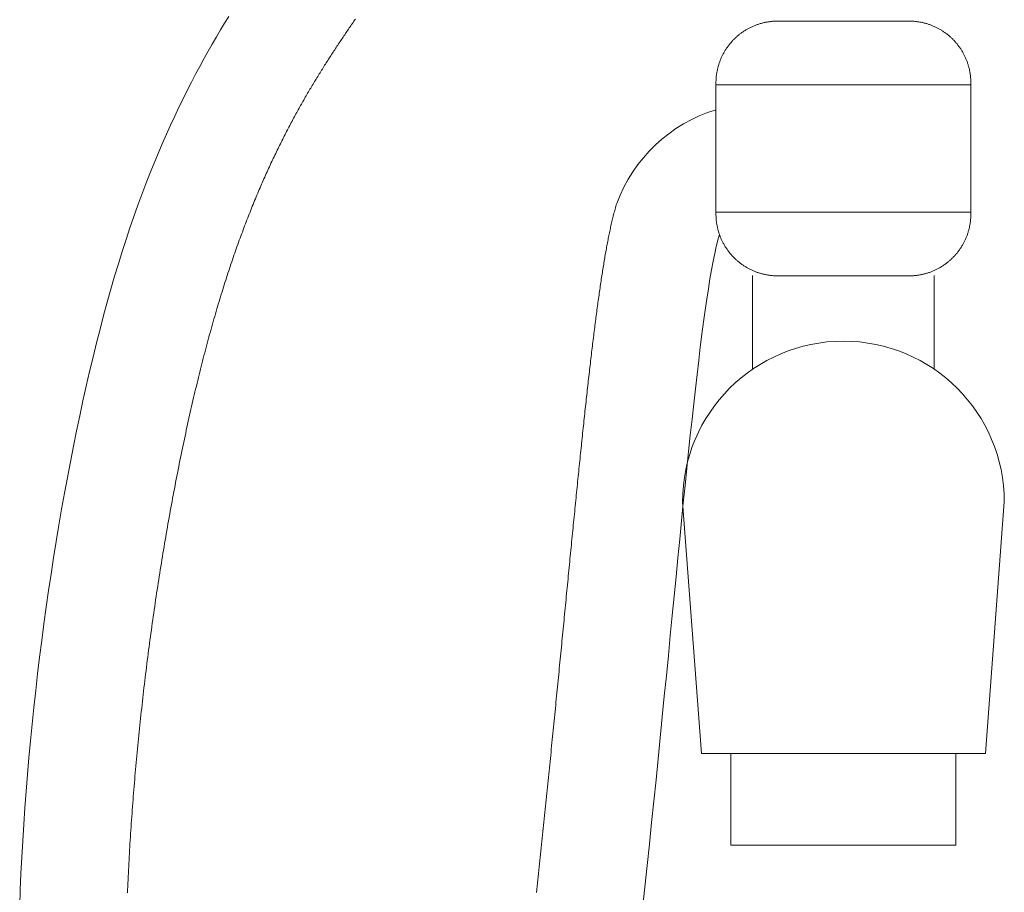
# Model space of a CAD drawing. Units: inches. Extents: x 64 to 1167, y 117 to 939.
# Tile 31 of 56: x 1044.26 to 1050.377, y 448.409 to 453.834. Entities that reach past the tile are written whole.
import ezdxf

# ---------------------------------------------------------------- set-up
doc = ezdxf.new("R2010")
doc.units = ezdxf.units.IN
doc.header["$MEASUREMENT"] = 0
doc.layers.add('A-FLOR-FIXT', color=8, linetype='Continuous', lineweight=18)

# ---------------------------------------------------------------- blocks, each defined once
blk = doc.blocks.new('A$C01277C2D')
for p, q in [((4.1384, 8.1142), (3.5444, 8.1142)), ((4.4355, 7.8172), (3.2473, 7.8172)), ((3.2473, 7.8172), (3.2473, 7.2231)), ((4.4355, 7.2231), (4.4355, 7.8172)), ((3.2473, 7.2231), (4.4355, 7.2231)), ((3.4178, 6.4903), (3.4178, 6.9283)), ((3.5444, 6.9261), (4.1384, 6.9261)), ((4.265, 6.4903), (4.265, 6.9283)), ((3.0914, 5.8714), (3.1791, 4.6978)), ((4.5914, 5.8714), (4.5038, 4.6978)), ((3.1791, 4.6978), (4.5038, 4.6978)), ((3.3169, 4.271), (3.3169, 4.6978)), ((4.366, 4.271), (4.366, 4.6978)), ((3.3169, 4.271), (4.366, 4.271))]:
    blk.add_line(p, q)
for points in [[(3.2634, 7.1191, 0), (3.2561, 7.0931, 0), (3.2487, 7.0635, 0), (3.2414, 7.0306, 0), (3.234, 6.9943, 0), (3.2267, 6.9547, 0), (3.2193, 6.912, 0), (3.2119, 6.8662, 0), (3.2044, 6.8175, 0), (3.197, 6.7657, 0), (3.1895, 6.7112, 0), (3.1819, 6.6539, 0), (3.1743, 6.594, 0), (3.1667, 6.5315, 0), (3.159, 6.4665, 0), (3.1512, 6.399, 0), (3.1434, 6.3293, 0), (3.1355, 6.2573, 0), (3.1276, 6.1831, 0), (3.1195, 6.1069, 0), (3.1114, 6.0287, 0), (3.1033, 5.9486, 0), (3.095, 5.8666, 0), (3.0866, 5.7829, 0), (3.0781, 5.6976, 0), (3.0696, 5.6107, 0), (3.0609, 5.5222, 0), (3.0522, 5.4324, 0), (3.0433, 5.3413, 0), (3.0343, 5.2489, 0), (3.0252, 5.1554, 0), (3.0159, 5.0608, 0), (3.0065, 4.9653, 0), (2.9971, 4.8688, 0), (2.9874, 4.7715, 0), (2.9776, 4.6735, 0), (2.9677, 4.5748, 0), (2.9577, 4.4756, 0), (2.9474, 4.3758, 0), (2.9371, 4.2757, 0), (2.9265, 4.1753, 0), (2.9158, 4.0746, 0), (2.9049, 3.9738, 0)], [(0.0012, 3.9867, 0), (0.004, 4.0619, 0), (0.0072, 4.1376, 0), (0.011, 4.2138, 0), (0.0153, 4.2904, 0), (0.0201, 4.3674, 0), (0.0254, 4.4448, 0), (0.0312, 4.5224, 0), (0.0375, 4.6002, 0), (0.0443, 4.6783, 0), (0.0515, 4.7564, 0), (0.0592, 4.8347, 0), (0.0673, 4.9129, 0), (0.0759, 4.9912, 0), (0.0849, 5.0694, 0), (0.0943, 5.1475, 0), (0.1041, 5.2255, 0), (0.1144, 5.3032, 0), (0.125, 5.3807, 0), (0.1361, 5.4579, 0), (0.1475, 5.5347, 0), (0.1593, 5.6112, 0), (0.1715, 5.6872, 0), (0.184, 5.7627, 0), (0.1969, 5.8377, 0), (0.2101, 5.9121, 0), (0.2237, 5.9858, 0), (0.2375, 6.0589, 0), (0.2517, 6.1312, 0), (0.2663, 6.2027, 0), (0.2811, 6.2734, 0), (0.2962, 6.3433, 0), (0.3116, 6.4122, 0), (0.3272, 6.4801, 0), (0.3432, 6.547, 0), (0.3594, 6.6129, 0), (0.3758, 6.6776, 0), (0.3925, 6.7411, 0), (0.4095, 6.8035, 0), (0.4266, 6.8645, 0), (0.444, 6.9243, 0), (0.4616, 6.9827, 0), (0.4794, 7.0398, 0), (0.4974, 7.0955, 0), (0.5155, 7.15, 0), (0.5339, 7.2032, 0), (0.5524, 7.2552, 0), (0.571, 7.3059, 0), (0.5898, 7.3555, 0), (0.6086, 7.4039, 0), (0.6276, 7.4512, 0), (0.6467, 7.4973, 0), (0.6659, 7.5424, 0), (0.6852, 7.5864, 0), (0.7045, 7.6293, 0), (0.7239, 7.6713, 0), (0.7433, 7.7122, 0), (0.7628, 7.7522, 0), (0.7822, 7.7913, 0), (0.8017, 7.8294, 0), (0.8212, 7.8667, 0), (0.8407, 7.9031, 0), (0.8601, 7.9386, 0), (0.8795, 7.9734, 0), (0.8989, 8.0074, 0), (0.9182, 8.0405, 0), (0.9374, 8.073, 0), (0.9566, 8.1047, 0), (0.9757, 8.1358, 0)], [(0.5038, 4.0475, 0), (0.5044, 4.0627, 0), (0.5051, 4.078, 0), (0.5057, 4.0932, 0), (0.5064, 4.1085, 0), (0.5071, 4.1238, 0), (0.5079, 4.1391, 0), (0.5086, 4.1545, 0), (0.5094, 4.1698, 0), (0.5102, 4.1852, 0), (0.511, 4.2007, 0), (0.5119, 4.2161, 0), (0.5127, 4.2316, 0), (0.5136, 4.2471, 0), (0.5145, 4.2626, 0), (0.5155, 4.2781, 0), (0.5164, 4.2937, 0), (0.5174, 4.3092, 0), (0.5184, 4.3248, 0), (0.5194, 4.3404, 0), (0.5205, 4.356, 0), (0.5215, 4.3717, 0), (0.5226, 4.3873, 0), (0.5237, 4.403, 0), (0.5249, 4.4187, 0), (0.526, 4.4344, 0), (0.5272, 4.4501, 0), (0.5284, 4.4658, 0), (0.5296, 4.4815, 0), (0.5308, 4.4973, 0), (0.5321, 4.513, 0), (0.5333, 4.5288, 0), (0.5346, 4.5446, 0), (0.5359, 4.5604, 0), (0.5373, 4.5762, 0), (0.5386, 4.592, 0), (0.54, 4.6078, 0), (0.5414, 4.6237, 0), (0.5428, 4.6395, 0), (0.5443, 4.6554, 0), (0.5457, 4.6712, 0), (0.5472, 4.6871, 0), (0.5487, 4.703, 0), (0.5502, 4.7188, 0), (0.5517, 4.7347, 0), (0.5533, 4.7506, 0), (0.5549, 4.7665, 0), (0.5564, 4.7824, 0), (0.5581, 4.7983, 0), (0.5597, 4.8141, 0), (0.5613, 4.83, 0), (0.563, 4.8459, 0), (0.5647, 4.8618, 0), (0.5664, 4.8777, 0), (0.5681, 4.8937, 0), (0.5699, 4.9096, 0), (0.5716, 4.9254, 0), (0.5734, 4.9413, 0), (0.5752, 4.9572, 0), (0.577, 4.9731, 0), (0.5789, 4.989, 0), (0.5807, 5.0049, 0), (0.5826, 5.0208, 0), (0.5845, 5.0367, 0), (0.5864, 5.0526, 0), (0.5883, 5.0684, 0), (0.5903, 5.0843, 0), (0.5922, 5.1001, 0), (0.5942, 5.116, 0), (0.5962, 5.1318, 0), (0.5982, 5.1477, 0), (0.6003, 5.1635, 0), (0.6023, 5.1793, 0), (0.6044, 5.1951, 0), (0.6065, 5.2109, 0), (0.6086, 5.2267, 0), (0.6107, 5.2425, 0), (0.6128, 5.2582, 0), (0.615, 5.274, 0), (0.6172, 5.2897, 0), (0.6194, 5.3055, 0), (0.6216, 5.3212, 0), (0.6238, 5.3369, 0), (0.626, 5.3525, 0), (0.6283, 5.3682, 0), (0.6306, 5.3839, 0), (0.6328, 5.3995, 0), (0.6351, 5.4151, 0), (0.6375, 5.4307, 0), (0.6398, 5.4463, 0), (0.6422, 5.4619, 0), (0.6445, 5.4775, 0), (0.6469, 5.493, 0), (0.6493, 5.5085, 0), (0.6517, 5.524, 0), (0.6542, 5.5395, 0), (0.6566, 5.5549, 0), (0.6591, 5.5704, 0), (0.6616, 5.5858, 0), (0.664, 5.6012, 0), (0.6666, 5.6165, 0), (0.6691, 5.6319, 0), (0.6716, 5.6472, 0), (0.6742, 5.6625, 0), (0.6767, 5.6778, 0), (0.6793, 5.693, 0), (0.6819, 5.7082, 0), (0.6845, 5.7234, 0), (0.6872, 5.7386, 0), (0.6898, 5.7537, 0), (0.6925, 5.7688, 0), (0.6951, 5.7839, 0), (0.6978, 5.799, 0), (0.7005, 5.814, 0), (0.7032, 5.829, 0), (0.7059, 5.8439, 0), (0.7087, 5.8589, 0), (0.7114, 5.8738, 0), (0.7142, 5.8886, 0), (0.717, 5.9035, 0), (0.7197, 5.9183, 0), (0.7225, 5.933, 0), (0.7254, 5.9478, 0), (0.7282, 5.9625, 0), (0.731, 5.9771, 0), (0.7339, 5.9918, 0), (0.7368, 6.0064, 0), (0.7396, 6.0209, 0), (0.7425, 6.0354, 0), (0.7454, 6.0499, 0), (0.7483, 6.0644, 0), (0.7513, 6.0788, 0), (0.7542, 6.0931, 0), (0.7572, 6.1075, 0), (0.7601, 6.1217, 0), (0.7631, 6.136, 0), (0.7661, 6.1502, 0), (0.7691, 6.1643, 0), (0.7721, 6.1785, 0), (0.7751, 6.1925, 0), (0.7781, 6.2066, 0), (0.7812, 6.2206, 0), (0.7842, 6.2345, 0), (0.7873, 6.2484, 0), (0.7904, 6.2622, 0), (0.7934, 6.2761, 0), (0.7965, 6.2898, 0), (0.7996, 6.3035, 0), (0.8027, 6.3172, 0), (0.8059, 6.3308, 0), (0.809, 6.3444, 0), (0.8122, 6.3579, 0), (0.8153, 6.3714, 0), (0.8185, 6.3848, 0), (0.8216, 6.3982, 0), (0.8248, 6.4115, 0), (0.828, 6.4247, 0), (0.8312, 6.4379, 0), (0.8344, 6.4511, 0), (0.8377, 6.4642, 0), (0.8409, 6.4772, 0), (0.8441, 6.4902, 0), (0.8474, 6.5031, 0), (0.8506, 6.516, 0), (0.8539, 6.5287, 0), (0.8571, 6.5415, 0), (0.8604, 6.5541, 0), (0.8637, 6.5667, 0), (0.867, 6.5793, 0), (0.8703, 6.5917, 0), (0.8736, 6.6042, 0), (0.8769, 6.6165, 0), (0.8802, 6.6288, 0), (0.8835, 6.6411, 0), (0.8869, 6.6532, 0), (0.8902, 6.6654, 0), (0.8935, 6.6774, 0), (0.8969, 6.6894, 0), (0.9002, 6.7013, 0), (0.9036, 6.7132, 0), (0.907, 6.7251, 0), (0.9104, 6.7368, 0), (0.9137, 6.7485, 0), (0.9171, 6.7602, 0), (0.9205, 6.7717, 0), (0.9239, 6.7832, 0), (0.9273, 6.7947, 0), (0.9308, 6.8061, 0), (0.9342, 6.8175, 0), (0.9376, 6.8287, 0), (0.941, 6.8399, 0), (0.9445, 6.8511, 0), (0.9479, 6.8622, 0), (0.9514, 6.8733, 0), (0.9548, 6.8843, 0), (0.9583, 6.8952, 0), (0.9618, 6.906, 0), (0.9652, 6.9169, 0), (0.9687, 6.9276, 0), (0.9722, 6.9383, 0), (0.9757, 6.9489, 0), (0.9792, 6.9595, 0), (0.9827, 6.97, 0), (0.9862, 6.9805, 0), (0.9897, 6.9909, 0), (0.9932, 7.0012, 0), (0.9967, 7.0115, 0), (1.0002, 7.0218, 0), (1.0037, 7.0319, 0), (1.0073, 7.042, 0), (1.0108, 7.0521, 0), (1.0143, 7.0621, 0), (1.0179, 7.072, 0), (1.0214, 7.0819, 0), (1.025, 7.0918, 0), (1.0285, 7.1015, 0), (1.0321, 7.1112, 0), (1.0356, 7.1209, 0), (1.0392, 7.1305, 0), (1.0428, 7.14, 0), (1.0463, 7.1495, 0), (1.0499, 7.159, 0), (1.0535, 7.1683, 0), (1.0571, 7.1777, 0), (1.0607, 7.187, 0), (1.0642, 7.1962, 0), (1.0678, 7.2054, 0), (1.0714, 7.2145, 0), (1.075, 7.2236, 0), (1.0786, 7.2326, 0), (1.0822, 7.2416, 0), (1.0858, 7.2505, 0), (1.0894, 7.2594, 0), (1.093, 7.2683, 0), (1.0966, 7.277, 0), (1.1002, 7.2858, 0), (1.1038, 7.2945, 0), (1.1075, 7.3031, 0), (1.1111, 7.3117, 0), (1.1147, 7.3203, 0), (1.1183, 7.3288, 0), (1.1219, 7.3372, 0), (1.1256, 7.3456, 0), (1.1292, 7.354, 0), (1.1328, 7.3623, 0), (1.1364, 7.3706, 0), (1.1401, 7.3788, 0), (1.1437, 7.387, 0), (1.1473, 7.3951, 0), (1.151, 7.4032, 0), (1.1546, 7.4113, 0), (1.1582, 7.4193, 0), (1.1619, 7.4273, 0), (1.1655, 7.4352, 0), (1.1691, 7.4431, 0), (1.1728, 7.4509, 0), (1.1764, 7.4587, 0), (1.1801, 7.4665, 0), (1.1837, 7.4742, 0), (1.1873, 7.4819, 0), (1.191, 7.4895, 0), (1.1946, 7.4971, 0), (1.1983, 7.5046, 0), (1.2019, 7.5122, 0), (1.2056, 7.5196, 0), (1.2092, 7.5271, 0), (1.2128, 7.5345, 0), (1.2165, 7.5418, 0), (1.2201, 7.5492, 0), (1.2238, 7.5564, 0), (1.2274, 7.5637, 0), (1.2311, 7.5709, 0), (1.2347, 7.5781, 0), (1.2384, 7.5852, 0), (1.242, 7.5923, 0), (1.2456, 7.5994, 0), (1.2493, 7.6064, 0), (1.2529, 7.6134, 0), (1.2566, 7.6203, 0), (1.2602, 7.6273, 0), (1.2638, 7.6341, 0), (1.2675, 7.641, 0), (1.2711, 7.6478, 0), (1.2748, 7.6546, 0), (1.2784, 7.6614, 0), (1.282, 7.6681, 0), (1.2856, 7.6748, 0), (1.2893, 7.6814, 0), (1.2929, 7.688, 0), (1.2965, 7.6946, 0), (1.3002, 7.7012, 0), (1.3038, 7.7077, 0), (1.3074, 7.7142, 0), (1.3111, 7.7207, 0), (1.3147, 7.7271, 0), (1.3183, 7.7336, 0), (1.3219, 7.7399, 0), (1.3256, 7.7463, 0), (1.3292, 7.7526, 0), (1.3328, 7.7589, 0), (1.3364, 7.7652, 0), (1.34, 7.7714, 0), (1.3437, 7.7776, 0), (1.3473, 7.7838, 0), (1.3509, 7.79, 0), (1.3545, 7.7961, 0), (1.3581, 7.8022, 0), (1.3617, 7.8083, 0), (1.3653, 7.8143, 0), (1.3689, 7.8204, 0), (1.3726, 7.8264, 0), (1.3762, 7.8324, 0), (1.3798, 7.8383, 0), (1.3834, 7.8442, 0), (1.387, 7.8502, 0), (1.3906, 7.8561, 0), (1.3942, 7.8619, 0), (1.3978, 7.8678, 0), (1.4014, 7.8736, 0), (1.405, 7.8794, 0), (1.4086, 7.8852, 0), (1.4122, 7.8909, 0), (1.4158, 7.8967, 0), (1.4194, 7.9024, 0), (1.423, 7.9081, 0), (1.4266, 7.9138, 0), (1.4302, 7.9194, 0), (1.4338, 7.9251, 0), (1.4374, 7.9307, 0), (1.441, 7.9363, 0), (1.4446, 7.9419, 0), (1.4482, 7.9475, 0), (1.4518, 7.953, 0), (1.4554, 7.9586, 0), (1.459, 7.9641, 0), (1.4626, 7.9696, 0), (1.4661, 7.9751, 0), (1.4697, 7.9806, 0), (1.4733, 7.986, 0), (1.4769, 7.9915, 0), (1.4805, 7.9969, 0), (1.4841, 8.0023, 0), (1.4876, 8.0077, 0), (1.4912, 8.0131, 0), (1.4948, 8.0185, 0), (1.4984, 8.0239, 0), (1.502, 8.0292, 0), (1.5055, 8.0346, 0), (1.5091, 8.0399, 0), (1.5127, 8.0452, 0), (1.5163, 8.0505, 0), (1.5198, 8.0558, 0), (1.5234, 8.0611, 0), (1.527, 8.0664, 0), (1.5306, 8.0717, 0), (1.5341, 8.0769, 0), (1.5377, 8.0822, 0), (1.5413, 8.0874, 0), (1.5448, 8.0927, 0), (1.5484, 8.0979, 0), (1.552, 8.1031, 0), (1.5555, 8.1083, 0), (1.5591, 8.1135, 0), (1.5627, 8.1187, 0), (1.5662, 8.1239, 0)], [(3.2474, 7.8172, 0), (3.2473, 7.8209, 0), (3.2472, 7.8245, 0), (3.2472, 7.8282, 0), (3.2473, 7.8319, 0), (3.2474, 7.8356, 0), (3.2475, 7.8392, 0), (3.2477, 7.8429, 0), (3.248, 7.8466, 0), (3.2482, 7.8502, 0), (3.2486, 7.8539, 0), (3.2489, 7.8576, 0), (3.2494, 7.8612, 0), (3.2498, 7.8648, 0), (3.2504, 7.8685, 0), (3.2509, 7.8721, 0), (3.2515, 7.8758, 0), (3.2522, 7.8794, 0), (3.2529, 7.883, 0), (3.2536, 7.8866, 0), (3.2544, 7.8902, 0), (3.2553, 7.8937, 0), (3.2562, 7.8973, 0), (3.2571, 7.9009, 0), (3.2581, 7.9044, 0), (3.2591, 7.9079, 0), (3.2602, 7.9115, 0), (3.2613, 7.915, 0), (3.2624, 7.9185, 0), (3.2636, 7.9219, 0), (3.2649, 7.9254, 0), (3.2662, 7.9288, 0), (3.2675, 7.9323, 0), (3.2689, 7.9357, 0), (3.2703, 7.9391, 0), (3.2717, 7.9425, 0), (3.2732, 7.9458, 0), (3.2748, 7.9491, 0), (3.2764, 7.9524, 0), (3.278, 7.9558, 0), (3.2797, 7.959, 0), (3.2814, 7.9623, 0), (3.2832, 7.9655, 0), (3.285, 7.9687, 0), (3.2868, 7.9719, 0), (3.2887, 7.9751, 0), (3.2906, 7.9782, 0), (3.2926, 7.9813, 0), (3.2946, 7.9844, 0), (3.2966, 7.9874, 0), (3.2987, 7.9905, 0), (3.3008, 7.9935, 0), (3.303, 7.9965, 0), (3.3051, 7.9994, 0), (3.3074, 8.0023, 0), (3.3096, 8.0052, 0), (3.3119, 8.0081, 0), (3.3143, 8.0109, 0), (3.3167, 8.0137, 0), (3.3191, 8.0165, 0), (3.3215, 8.0193, 0), (3.324, 8.022, 0), (3.3265, 8.0247, 0), (3.3291, 8.0273, 0), (3.3316, 8.0299, 0), (3.3343, 8.0325, 0), (3.3369, 8.0351, 0), (3.3396, 8.0376, 0), (3.3423, 8.0401, 0), (3.3451, 8.0425, 0), (3.3478, 8.0449, 0), (3.3506, 8.0473, 0), (3.3535, 8.0496, 0), (3.3563, 8.0519, 0), (3.3592, 8.0542, 0), (3.3622, 8.0564, 0), (3.3651, 8.0586, 0), (3.3681, 8.0608, 0), (3.3711, 8.0629, 0), (3.3741, 8.065, 0), (3.3772, 8.067, 0), (3.3803, 8.069, 0), (3.3834, 8.071, 0), (3.3865, 8.0729, 0), (3.3897, 8.0748, 0), (3.3929, 8.0766, 0), (3.3961, 8.0784, 0), (3.3993, 8.0802, 0), (3.4026, 8.0819, 0), (3.4058, 8.0836, 0), (3.4091, 8.0852, 0), (3.4124, 8.0868, 0), (3.4158, 8.0883, 0), (3.4191, 8.0898, 0), (3.4225, 8.0913, 0), (3.4259, 8.0927, 0), (3.4293, 8.0941, 0), (3.4327, 8.0954, 0), (3.4362, 8.0967, 0), (3.4396, 8.098, 0), (3.4431, 8.0991, 0), (3.4466, 8.1003, 0), (3.4501, 8.1014, 0), (3.4536, 8.1025, 0), (3.4572, 8.1035, 0), (3.4607, 8.1045, 0), (3.4643, 8.1054, 0), (3.4678, 8.1063, 0), (3.4714, 8.1071, 0), (3.475, 8.1079, 0), (3.4786, 8.1087, 0), (3.4822, 8.1094, 0), (3.4858, 8.11, 0), (3.4895, 8.1106, 0), (3.4931, 8.1112, 0), (3.4967, 8.1117, 0), (3.5004, 8.1122, 0), (3.504, 8.1126, 0), (3.5077, 8.113, 0), (3.5113, 8.1133, 0), (3.515, 8.1136, 0), (3.5187, 8.1139, 0), (3.5223, 8.1141, 0), (3.526, 8.1142, 0), (3.5297, 8.1143, 0), (3.5334, 8.1143, 0), (3.537, 8.1143, 0), (3.5407, 8.1143, 0), (3.5444, 8.1142, 0)], [(4.1384, 8.1142, 0), (4.1421, 8.1143, 0), (4.1458, 8.1143, 0), (4.1494, 8.1143, 0), (4.1531, 8.1143, 0), (4.1568, 8.1142, 0), (4.1605, 8.1141, 0), (4.1641, 8.1139, 0), (4.1678, 8.1136, 0), (4.1715, 8.1133, 0), (4.1751, 8.113, 0), (4.1788, 8.1126, 0), (4.1825, 8.1122, 0), (4.1861, 8.1117, 0), (4.1897, 8.1112, 0), (4.1934, 8.1106, 0), (4.197, 8.11, 0), (4.2006, 8.1094, 0), (4.2042, 8.1087, 0), (4.2078, 8.1079, 0), (4.2114, 8.1071, 0), (4.215, 8.1063, 0), (4.2186, 8.1054, 0), (4.2221, 8.1045, 0), (4.2257, 8.1035, 0), (4.2292, 8.1025, 0), (4.2327, 8.1014, 0), (4.2362, 8.1003, 0), (4.2397, 8.0991, 0), (4.2432, 8.098, 0), (4.2466, 8.0967, 0), (4.2501, 8.0954, 0), (4.2535, 8.0941, 0), (4.2569, 8.0927, 0), (4.2603, 8.0913, 0), (4.2637, 8.0898, 0), (4.267, 8.0883, 0), (4.2704, 8.0868, 0), (4.2737, 8.0852, 0), (4.277, 8.0836, 0), (4.2803, 8.0819, 0), (4.2835, 8.0802, 0), (4.2867, 8.0784, 0), (4.29, 8.0766, 0), (4.2931, 8.0748, 0), (4.2963, 8.0729, 0), (4.2994, 8.071, 0), (4.3025, 8.069, 0), (4.3056, 8.067, 0), (4.3087, 8.065, 0), (4.3117, 8.0629, 0), (4.3147, 8.0608, 0), (4.3177, 8.0586, 0), (4.3207, 8.0564, 0), (4.3236, 8.0542, 0), (4.3265, 8.0519, 0), (4.3293, 8.0496, 0), (4.3322, 8.0473, 0), (4.335, 8.0449, 0), (4.3378, 8.0425, 0), (4.3405, 8.0401, 0), (4.3432, 8.0376, 0), (4.3459, 8.0351, 0), (4.3486, 8.0325, 0), (4.3512, 8.0299, 0), (4.3537, 8.0273, 0), (4.3563, 8.0247, 0), (4.3588, 8.022, 0), (4.3613, 8.0193, 0), (4.3637, 8.0165, 0), (4.3662, 8.0137, 0), (4.3685, 8.0109, 0), (4.3709, 8.0081, 0), (4.3732, 8.0052, 0), (4.3754, 8.0023, 0), (4.3777, 7.9994, 0), (4.3799, 7.9965, 0), (4.382, 7.9935, 0), (4.3841, 7.9905, 0), (4.3862, 7.9874, 0), (4.3882, 7.9844, 0), (4.3902, 7.9813, 0), (4.3922, 7.9782, 0), (4.3941, 7.9751, 0), (4.396, 7.9719, 0), (4.3978, 7.9687, 0), (4.3996, 7.9655, 0), (4.4014, 7.9623, 0), (4.4031, 7.959, 0), (4.4048, 7.9558, 0), (4.4064, 7.9524, 0), (4.408, 7.9491, 0), (4.4096, 7.9458, 0), (4.4111, 7.9425, 0), (4.4125, 7.9391, 0), (4.4139, 7.9357, 0), (4.4153, 7.9323, 0), (4.4167, 7.9288, 0), (4.4179, 7.9254, 0), (4.4192, 7.9219, 0), (4.4204, 7.9185, 0), (4.4215, 7.915, 0), (4.4227, 7.9115, 0), (4.4237, 7.9079, 0), (4.4247, 7.9044, 0), (4.4257, 7.9009, 0), (4.4267, 7.8973, 0), (4.4275, 7.8937, 0), (4.4284, 7.8902, 0), (4.4292, 7.8866, 0), (4.4299, 7.883, 0), (4.4306, 7.8794, 0), (4.4313, 7.8758, 0), (4.4319, 7.8721, 0), (4.4325, 7.8685, 0), (4.433, 7.8648, 0), (4.4334, 7.8612, 0), (4.4339, 7.8576, 0), (4.4342, 7.8539, 0), (4.4346, 7.8502, 0), (4.4349, 7.8466, 0), (4.4351, 7.8429, 0), (4.4353, 7.8392, 0), (4.4354, 7.8356, 0), (4.4355, 7.8319, 0), (4.4356, 7.8282, 0), (4.4356, 7.8245, 0), (4.4355, 7.8209, 0), (4.4355, 7.8172, 0)], [(2.7847, 7.2636, 0), (2.7827, 7.257, 0), (2.7808, 7.2505, 0), (2.7789, 7.244, 0), (2.7771, 7.2375, 0), (2.7753, 7.231, 0), (2.7735, 7.2245, 0), (2.7718, 7.2181, 0), (2.7701, 7.2116, 0), (2.7685, 7.2052, 0), (2.7668, 7.1988, 0), (2.7652, 7.1923, 0), (2.7637, 7.1859, 0), (2.7621, 7.1794, 0), (2.7606, 7.173, 0), (2.7591, 7.1665, 0), (2.7576, 7.16, 0), (2.7562, 7.1535, 0), (2.7548, 7.147, 0), (2.7534, 7.1405, 0), (2.752, 7.1339, 0), (2.7506, 7.1274, 0), (2.7493, 7.1208, 0), (2.7479, 7.1141, 0), (2.7466, 7.1075, 0), (2.7453, 7.1008, 0), (2.744, 7.0941, 0), (2.7427, 7.0873, 0), (2.7414, 7.0805, 0), (2.7401, 7.0736, 0), (2.7388, 7.0667, 0), (2.7376, 7.0597, 0), (2.7363, 7.0527, 0), (2.735, 7.0457, 0), (2.7337, 7.0386, 0), (2.7325, 7.0314, 0), (2.7312, 7.0242, 0), (2.7299, 7.0169, 0), (2.7287, 7.0096, 0), (2.7274, 7.0023, 0), (2.7262, 6.9949, 0), (2.725, 6.9874, 0), (2.7237, 6.9799, 0), (2.7225, 6.9724, 0), (2.7212, 6.9648, 0), (2.72, 6.9571, 0), (2.7188, 6.9494, 0), (2.7176, 6.9417, 0), (2.7164, 6.9339, 0), (2.7152, 6.926, 0), (2.714, 6.9181, 0), (2.7127, 6.9102, 0), (2.7115, 6.9022, 0), (2.7103, 6.8941, 0), (2.7091, 6.886, 0), (2.7079, 6.8778, 0), (2.7067, 6.8696, 0), (2.7055, 6.8614, 0), (2.7043, 6.8531, 0), (2.7032, 6.8447, 0), (2.702, 6.8363, 0), (2.7008, 6.8278, 0), (2.6996, 6.8193, 0), (2.6984, 6.8107, 0), (2.6972, 6.8021, 0), (2.696, 6.7934, 0), (2.6949, 6.7847, 0), (2.6937, 6.7759, 0), (2.6925, 6.7671, 0), (2.6913, 6.7582, 0), (2.6901, 6.7492, 0), (2.6889, 6.7402, 0), (2.6877, 6.7312, 0), (2.6866, 6.722, 0), (2.6854, 6.7129, 0), (2.6842, 6.7037, 0), (2.683, 6.6944, 0), (2.6818, 6.6851, 0), (2.6806, 6.6757, 0), (2.6795, 6.6663, 0), (2.6783, 6.6568, 0), (2.6771, 6.6473, 0), (2.6759, 6.6377, 0), (2.6747, 6.6281, 0), (2.6735, 6.6184, 0), (2.6723, 6.6087, 0), (2.6712, 6.5989, 0), (2.67, 6.5891, 0), (2.6688, 6.5792, 0), (2.6676, 6.5693, 0), (2.6664, 6.5593, 0), (2.6652, 6.5493, 0), (2.6641, 6.5392, 0), (2.6629, 6.5291, 0), (2.6617, 6.5189, 0), (2.6605, 6.5087, 0), (2.6593, 6.4984, 0), (2.6581, 6.4881, 0), (2.6569, 6.4777, 0), (2.6557, 6.4673, 0), (2.6545, 6.4568, 0), (2.6534, 6.4463, 0), (2.6522, 6.4358, 0), (2.651, 6.4252, 0), (2.6498, 6.4145, 0), (2.6486, 6.4038, 0), (2.6474, 6.3931, 0), (2.6462, 6.3823, 0), (2.645, 6.3715, 0), (2.6438, 6.3606, 0), (2.6426, 6.3496, 0), (2.6414, 6.3387, 0), (2.6402, 6.3277, 0), (2.639, 6.3166, 0), (2.6378, 6.3055, 0), (2.6366, 6.2943, 0), (2.6354, 6.2832, 0), (2.6342, 6.2719, 0), (2.633, 6.2606, 0), (2.6318, 6.2493, 0), (2.6306, 6.2379, 0), (2.6294, 6.2265, 0), (2.6281, 6.2151, 0), (2.6269, 6.2036, 0), (2.6257, 6.192, 0), (2.6245, 6.1805, 0), (2.6233, 6.1688, 0), (2.6221, 6.1571, 0), (2.6208, 6.1454, 0), (2.6196, 6.1337, 0), (2.6184, 6.1219, 0), (2.6172, 6.1101, 0), (2.6159, 6.0982, 0), (2.6147, 6.0863, 0), (2.6135, 6.0743, 0), (2.6122, 6.0623, 0), (2.611, 6.0503, 0), (2.6098, 6.0382, 0), (2.6086, 6.0261, 0), (2.6073, 6.0139, 0), (2.6061, 6.0017, 0), (2.6048, 5.9895, 0), (2.6036, 5.9772, 0), (2.6023, 5.9649, 0), (2.6011, 5.9525, 0), (2.5998, 5.9402, 0), (2.5986, 5.9277, 0), (2.5973, 5.9153, 0), (2.5961, 5.9028, 0), (2.5948, 5.8902, 0), (2.5936, 5.8776, 0), (2.5923, 5.865, 0), (2.5911, 5.8524, 0), (2.5898, 5.8397, 0), (2.5885, 5.827, 0), (2.5873, 5.8142, 0), (2.586, 5.8014, 0), (2.5847, 5.7886, 0), (2.5834, 5.7757, 0), (2.5822, 5.7629, 0), (2.5809, 5.7499, 0), (2.5796, 5.737, 0), (2.5783, 5.724, 0), (2.577, 5.711, 0), (2.5758, 5.6979, 0), (2.5745, 5.6848, 0), (2.5732, 5.6717, 0), (2.5719, 5.6585, 0), (2.5706, 5.6453, 0), (2.5693, 5.6321, 0), (2.568, 5.6189, 0), (2.5667, 5.6056, 0), (2.5654, 5.5923, 0), (2.5641, 5.5789, 0), (2.5628, 5.5656, 0), (2.5615, 5.5522, 0), (2.5602, 5.5387, 0), (2.5588, 5.5253, 0), (2.5575, 5.5118, 0), (2.5562, 5.4983, 0), (2.5549, 5.4847, 0), (2.5536, 5.4712, 0), (2.5522, 5.4576, 0), (2.5509, 5.4439, 0), (2.5496, 5.4303, 0), (2.5482, 5.4166, 0), (2.5469, 5.4029, 0), (2.5456, 5.3891, 0), (2.5442, 5.3754, 0), (2.5429, 5.3616, 0), (2.5415, 5.3478, 0), (2.5402, 5.334, 0), (2.5388, 5.3201, 0), (2.5375, 5.3062, 0), (2.5361, 5.2923, 0), (2.5348, 5.2784, 0), (2.5334, 5.2644, 0), (2.532, 5.2504, 0), (2.5307, 5.2364, 0), (2.5293, 5.2224, 0), (2.528, 5.2083, 0), (2.5266, 5.1942, 0), (2.5252, 5.1801, 0), (2.5238, 5.166, 0), (2.5224, 5.1519, 0), (2.521, 5.1377, 0), (2.5197, 5.1235, 0), (2.5183, 5.1093, 0), (2.5169, 5.0951, 0), (2.5155, 5.0808, 0), (2.5141, 5.0666, 0), (2.5127, 5.0523, 0), (2.5113, 5.038, 0), (2.5099, 5.0237, 0), (2.5085, 5.0093, 0), (2.5071, 4.995, 0), (2.5057, 4.9806, 0), (2.5042, 4.9662, 0), (2.5028, 4.9517, 0), (2.5014, 4.9373, 0), (2.5, 4.9229, 0), (2.4985, 4.9084, 0), (2.4971, 4.8939, 0), (2.4957, 4.8794, 0), (2.4942, 4.8649, 0), (2.4928, 4.8503, 0), (2.4913, 4.8358, 0), (2.4899, 4.8212, 0), (2.4884, 4.8066, 0), (2.487, 4.792, 0), (2.4855, 4.7774, 0), (2.4841, 4.7627, 0), (2.4826, 4.7481, 0), (2.4811, 4.7335, 0), (2.4797, 4.7188, 0), (2.4782, 4.7041, 0), (2.4767, 4.6894, 0), (2.4752, 4.6747, 0), (2.4738, 4.66, 0), (2.4723, 4.6452, 0), (2.4708, 4.6305, 0), (2.4693, 4.6157, 0), (2.4678, 4.6009, 0), (2.4663, 4.5861, 0), (2.4648, 4.5713, 0), (2.4633, 4.5565, 0), (2.4618, 4.5417, 0), (2.4603, 4.5269, 0), (2.4588, 4.5121, 0), (2.4573, 4.4972, 0), (2.4557, 4.4824, 0), (2.4542, 4.4675, 0), (2.4527, 4.4526, 0), (2.4511, 4.4378, 0), (2.4496, 4.4229, 0), (2.4481, 4.408, 0), (2.4465, 4.3931, 0), (2.445, 4.3782, 0), (2.4434, 4.3632, 0), (2.4419, 4.3483, 0), (2.4403, 4.3334, 0), (2.4388, 4.3185, 0), (2.4372, 4.3035, 0), (2.4356, 4.2886, 0), (2.4341, 4.2736, 0), (2.4325, 4.2587, 0), (2.4309, 4.2437, 0), (2.4293, 4.2287, 0), (2.4278, 4.2138, 0), (2.4262, 4.1988, 0), (2.4246, 4.1838, 0), (2.423, 4.1689, 0), (2.4214, 4.1539, 0), (2.4198, 4.1389, 0), (2.4182, 4.1239, 0), (2.4166, 4.1089, 0), (2.415, 4.0939, 0), (2.4133, 4.0789, 0), (2.4117, 4.064, 0), (2.4101, 4.049, 0)], [(3.5444, 6.9261, 0), (3.5407, 6.926, 0), (3.537, 6.926, 0), (3.5334, 6.926, 0), (3.5297, 6.9261, 0), (3.526, 6.9261, 0), (3.5223, 6.9263, 0), (3.5187, 6.9265, 0), (3.515, 6.9267, 0), (3.5113, 6.927, 0), (3.5077, 6.9273, 0), (3.504, 6.9277, 0), (3.5004, 6.9281, 0), (3.4967, 6.9286, 0), (3.4931, 6.9291, 0), (3.4895, 6.9297, 0), (3.4858, 6.9303, 0), (3.4822, 6.931, 0), (3.4786, 6.9317, 0), (3.475, 6.9324, 0), (3.4714, 6.9332, 0), (3.4678, 6.934, 0), (3.4643, 6.9349, 0), (3.4607, 6.9359, 0), (3.4572, 6.9368, 0), (3.4536, 6.9379, 0), (3.4501, 6.9389, 0), (3.4466, 6.94, 0), (3.4431, 6.9412, 0), (3.4396, 6.9424, 0), (3.4362, 6.9436, 0), (3.4327, 6.9449, 0), (3.4293, 6.9463, 0), (3.4259, 6.9476, 0), (3.4225, 6.949, 0), (3.4191, 6.9505, 0), (3.4158, 6.952, 0), (3.4124, 6.9536, 0), (3.4091, 6.9552, 0), (3.4058, 6.9568, 0), (3.4026, 6.9585, 0), (3.3993, 6.9602, 0), (3.3961, 6.9619, 0), (3.3929, 6.9637, 0), (3.3897, 6.9656, 0), (3.3865, 6.9675, 0), (3.3834, 6.9694, 0), (3.3803, 6.9713, 0), (3.3772, 6.9733, 0), (3.3741, 6.9754, 0), (3.3711, 6.9775, 0), (3.3681, 6.9796, 0), (3.3651, 6.9817, 0), (3.3622, 6.9839, 0), (3.3592, 6.9861, 0), (3.3563, 6.9884, 0), (3.3535, 6.9907, 0), (3.3506, 6.9931, 0), (3.3478, 6.9954, 0), (3.3451, 6.9978, 0), (3.3423, 7.0003, 0), (3.3396, 7.0028, 0), (3.3369, 7.0053, 0), (3.3343, 7.0078, 0), (3.3316, 7.0104, 0), (3.3291, 7.013, 0), (3.3265, 7.0157, 0), (3.324, 7.0184, 0), (3.3215, 7.0211, 0), (3.3191, 7.0238, 0), (3.3167, 7.0266, 0), (3.3143, 7.0294, 0), (3.3119, 7.0322, 0), (3.3096, 7.0351, 0), (3.3074, 7.038, 0), (3.3051, 7.0409, 0), (3.303, 7.0439, 0), (3.3008, 7.0469, 0), (3.2987, 7.0499, 0), (3.2966, 7.0529, 0), (3.2946, 7.056, 0), (3.2926, 7.059, 0), (3.2906, 7.0621, 0), (3.2887, 7.0653, 0), (3.2868, 7.0685, 0), (3.285, 7.0716, 0), (3.2832, 7.0748, 0), (3.2814, 7.0781, 0), (3.2797, 7.0813, 0), (3.278, 7.0846, 0), (3.2764, 7.0879, 0), (3.2748, 7.0912, 0), (3.2732, 7.0945, 0), (3.2717, 7.0979, 0), (3.2703, 7.1013, 0), (3.2689, 7.1047, 0), (3.2675, 7.1081, 0), (3.2662, 7.1115, 0), (3.2649, 7.1149, 0), (3.2636, 7.1184, 0), (3.2624, 7.1219, 0), (3.2613, 7.1254, 0), (3.2602, 7.1289, 0), (3.2591, 7.1324, 0), (3.2581, 7.1359, 0), (3.2571, 7.1395, 0), (3.2562, 7.143, 0), (3.2553, 7.1466, 0), (3.2544, 7.1502, 0), (3.2536, 7.1538, 0), (3.2529, 7.1574, 0), (3.2522, 7.161, 0), (3.2515, 7.1646, 0), (3.2509, 7.1682, 0), (3.2504, 7.1718, 0), (3.2498, 7.1755, 0), (3.2494, 7.1791, 0), (3.2489, 7.1828, 0), (3.2486, 7.1864, 0), (3.2482, 7.1901, 0), (3.248, 7.1938, 0), (3.2477, 7.1974, 0), (3.2475, 7.2011, 0), (3.2474, 7.2048, 0), (3.2473, 7.2085, 0), (3.2472, 7.2121, 0), (3.2472, 7.2158, 0), (3.2473, 7.2195, 0), (3.2474, 7.2232, 0)], [(4.4355, 7.2232, 0), (4.4355, 7.2195, 0), (4.4356, 7.2158, 0), (4.4356, 7.2121, 0), (4.4355, 7.2085, 0), (4.4354, 7.2048, 0), (4.4353, 7.2011, 0), (4.4351, 7.1974, 0), (4.4349, 7.1938, 0), (4.4346, 7.1901, 0), (4.4342, 7.1864, 0), (4.4339, 7.1828, 0), (4.4334, 7.1791, 0), (4.433, 7.1755, 0), (4.4325, 7.1719, 0), (4.4319, 7.1682, 0), (4.4313, 7.1646, 0), (4.4306, 7.161, 0), (4.4299, 7.1574, 0), (4.4292, 7.1538, 0), (4.4284, 7.1502, 0), (4.4275, 7.1466, 0), (4.4267, 7.143, 0), (4.4257, 7.1395, 0), (4.4247, 7.1359, 0), (4.4237, 7.1324, 0), (4.4227, 7.1289, 0), (4.4215, 7.1254, 0), (4.4204, 7.1219, 0), (4.4192, 7.1184, 0), (4.4179, 7.1149, 0), (4.4167, 7.1115, 0), (4.4153, 7.1081, 0), (4.4139, 7.1047, 0), (4.4125, 7.1013, 0), (4.4111, 7.0979, 0), (4.4096, 7.0945, 0), (4.408, 7.0912, 0), (4.4064, 7.0879, 0), (4.4048, 7.0846, 0), (4.4031, 7.0813, 0), (4.4014, 7.0781, 0), (4.3996, 7.0748, 0), (4.3978, 7.0716, 0), (4.396, 7.0685, 0), (4.3941, 7.0653, 0), (4.3922, 7.0621, 0), (4.3902, 7.059, 0), (4.3882, 7.056, 0), (4.3862, 7.0529, 0), (4.3841, 7.0499, 0), (4.382, 7.0469, 0), (4.3799, 7.0439, 0), (4.3777, 7.0409, 0), (4.3754, 7.038, 0), (4.3732, 7.0351, 0), (4.3709, 7.0322, 0), (4.3685, 7.0294, 0), (4.3662, 7.0266, 0), (4.3637, 7.0238, 0), (4.3613, 7.0211, 0), (4.3588, 7.0184, 0), (4.3563, 7.0157, 0), (4.3537, 7.013, 0), (4.3512, 7.0104, 0), (4.3486, 7.0078, 0), (4.3459, 7.0053, 0), (4.3432, 7.0028, 0), (4.3405, 7.0003, 0), (4.3378, 6.9978, 0), (4.335, 6.9954, 0), (4.3322, 6.9931, 0), (4.3293, 6.9907, 0), (4.3265, 6.9884, 0), (4.3236, 6.9861, 0), (4.3207, 6.9839, 0), (4.3177, 6.9817, 0), (4.3147, 6.9796, 0), (4.3117, 6.9775, 0), (4.3087, 6.9754, 0), (4.3056, 6.9733, 0), (4.3025, 6.9713, 0), (4.2994, 6.9694, 0), (4.2963, 6.9675, 0), (4.2931, 6.9656, 0), (4.29, 6.9637, 0), (4.2867, 6.9619, 0), (4.2835, 6.9602, 0), (4.2803, 6.9585, 0), (4.277, 6.9568, 0), (4.2737, 6.9552, 0), (4.2704, 6.9536, 0), (4.267, 6.952, 0), (4.2637, 6.9505, 0), (4.2603, 6.949, 0), (4.2569, 6.9476, 0), (4.2535, 6.9463, 0), (4.2501, 6.9449, 0), (4.2466, 6.9436, 0), (4.2432, 6.9424, 0), (4.2397, 6.9412, 0), (4.2362, 6.94, 0), (4.2327, 6.9389, 0), (4.2292, 6.9379, 0), (4.2257, 6.9368, 0), (4.2221, 6.9359, 0), (4.2186, 6.9349, 0), (4.215, 6.934, 0), (4.2114, 6.9332, 0), (4.2078, 6.9324, 0), (4.2042, 6.9317, 0), (4.2006, 6.931, 0), (4.197, 6.9303, 0), (4.1934, 6.9297, 0), (4.1897, 6.9291, 0), (4.1861, 6.9286, 0), (4.1825, 6.9281, 0), (4.1788, 6.9277, 0), (4.1751, 6.9273, 0), (4.1715, 6.927, 0), (4.1678, 6.9267, 0), (4.1641, 6.9265, 0), (4.1605, 6.9263, 0), (4.1568, 6.9261, 0), (4.1531, 6.9261, 0), (4.1494, 6.926, 0), (4.1458, 6.926, 0), (4.1421, 6.926, 0), (4.1384, 6.9261, 0)]]:
    blk.add_polyline3d(points)
for centre, radius, start, end in [((3.4578, 7.0153), 0.7174, 107.056, 159.7504), ((3.8414, 5.8714), 0.75, 0, 180)]:
    blk.add_arc(centre, radius, start, end)

msp = doc.modelspace()

# ---------------------------------------------------------------- block references
at = {"layer": 'A-FLOR-FIXT', "xscale": 1.33257137012807, "yscale": 1.33257137012807, "zscale": 1.33257137012807}
msp.add_blockref('A$C01277C2D', (1044.2585, 443.012), dxfattribs=at)

doc.saveas('drawing.dxf')
